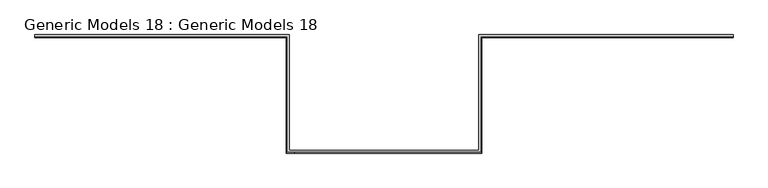
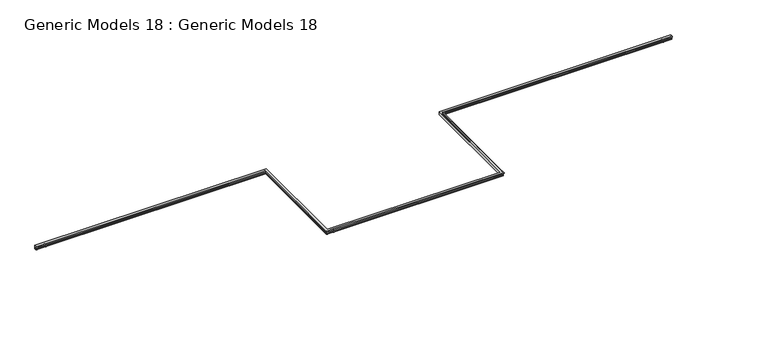
"""IFC4 building model written with IfcOpenShell, lengths in millimetres: proxy geometry, Generic Models 18 : Generic Models 18."""

from ifc_helpers import new_model, si_unit, frame, origin, place, context, project, spatial, circle_curve, ellipse_curve, source, transform, mapped, element, save
from ifc_brep_helpers import plane_surface, cylinder_surface, advanced_brep


def generic_models_18_generic_models_18_2a58dc35(model_context):
    return source(origin(), model_context, "Body", "AdvancedBrep", [
        advanced_brep(
        [(-8761.2825076, -5430.1542653, 7442.2), (-8761.2825076, -5379.3542653, 7442.2), (-8761.2825076, -5379.3542653, 7353.3), (-8761.2825076, -5417.4542653, 7353.3), (-8761.2825076, -5417.4542653, 7366.0), (-8761.2825076, -5417.4542653, 7378.7), (-8761.2825076, -5417.4542653, 7404.1), (-8761.2825076, -5417.4542653, 7416.8), (-8761.2825076, -5430.1542653, 7416.8), (-8532.6825076, -5430.1542653, 7442.2), (-3097.0825076, -5430.1542653, 7442.2), (-3097.0825076, -8034.2292912, 7442.2), (-2931.9825076, -8034.2292912, 7442.2), (1271.7174924, -8034.2292912, 7442.2), (1271.7174924, -7869.1292912, 7442.2), (1271.7174924, -5430.1542653, 7442.2), (6707.3174924, -5430.1542653, 7442.2), (6935.9174924, -5430.1542653, 7442.2), (6935.9174924, -5379.3542653, 7442.2), (1220.9174924, -5379.3542653, 7442.2), (1220.9174924, -7983.4292912, 7442.2), (-3046.2825076, -7983.4292912, 7442.2), (-3046.2825076, -5379.3542653, 7442.2), (-3046.2825076, -5379.3542653, 7353.3), (-3046.2825076, -7983.4292912, 7353.3), (1220.9174924, -7983.4292912, 7353.3), (1220.9174924, -5379.3542653, 7353.3), (6935.9174924, -5379.3542653, 7353.3), (6935.9174924, -5417.4542653, 7353.3), (6707.3174924, -5417.4542653, 7353.3), (1259.0174924, -5417.4542653, 7353.3), (1259.0174924, -7869.1292912, 7353.3), (1259.0174924, -8021.5292912, 7353.3), (-2931.9825076, -8021.5292912, 7353.3), (-3084.3825076, -8021.5292912, 7353.3), (-3084.3825076, -5417.4542653, 7353.3), (-8532.6825076, -5417.4542653, 7353.3), (-8532.6825076, -5417.4542653, 7366.0), (-3084.3825076, -5417.4542653, 7366.0), (-3084.3825076, -5417.4542653, 7378.7), (-8532.6825076, -5417.4542653, 7378.7), (-8532.6825076, -5417.4542653, 7404.1), (-3084.3825076, -5417.4542653, 7404.1), (-3084.3825076, -5417.4542653, 7416.8), (-3084.3825076, -8021.5292912, 7416.8), (1259.0174924, -8021.5292912, 7416.8), (1259.0174924, -5417.4542653, 7416.8), (6935.9174924, -5417.4542653, 7416.8), (6935.9174924, -5430.1542653, 7416.8), (6707.3174924, -5430.1542653, 7416.8), (1271.7174924, -5430.1542653, 7416.8), (1271.7174924, -7869.1292912, 7416.8), (1271.7174924, -8034.2292912, 7416.8), (-2931.9825076, -8034.2292912, 7416.8), (-3097.0825076, -8034.2292912, 7416.8), (-3097.0825076, -5430.1542653, 7416.8), (-8532.6825076, -5430.1542653, 7416.8), (-3084.3825076, -8021.5292912, 7366.0), (-3084.3825076, -8021.5292912, 7378.7), (-3084.3825076, -8021.5292912, 7404.1), (-2931.9825076, -8021.5292912, 7366.0), (1259.0174924, -8021.5292912, 7366.0), (1259.0174924, -8021.5292912, 7378.7), (-2931.9825076, -8021.5292912, 7378.7), (-2931.9825076, -8021.5292912, 7404.1), (1259.0174924, -8021.5292912, 7404.1), (1259.0174924, -7869.1292912, 7366.0), (1259.0174924, -5417.4542653, 7366.0), (1259.0174924, -5417.4542653, 7378.7), (1259.0174924, -7869.1292912, 7378.7), (1259.0174924, -7869.1292912, 7404.1), (1259.0174924, -5417.4542653, 7404.1), (6707.3174924, -5417.4542653, 7366.0), (6935.9174924, -5417.4542653, 7366.0), (6935.9174924, -5417.4542653, 7378.7), (6707.3174924, -5417.4542653, 7378.7), (6707.3174924, -5417.4542653, 7404.1), (6935.9174924, -5417.4542653, 7404.1)],
        [
            (0, 1),
            (1, 2),
            (2, 3),
            (3, 4, circle_curve(frame((-8761.2825076, -5421.1991851, 7359.65), z_axis=(-1.0, 0.0, 0.0), x_axis=(0.0, 1.0, 0.0)), 7.3720367)),
            (4, 5),
            (5, 6, circle_curve(frame((-8761.2825076, -5417.4542653, 7391.4), z_axis=(-1.0, 0.0, 0.0), x_axis=(0.0, 1.0, 0.0)), 12.7)),
            (6, 7),
            (7, 8),
            (8, 0, circle_curve(frame((-8761.2825076, -5430.1542653, 7429.5), z_axis=(-1.0, 0.0, 0.0), x_axis=(0.0, 1.0, 0.0)), 12.7)),
            (0, 9),
            (9, 10),
            (10, 11),
            (11, 12),
            (12, 13),
            (13, 14),
            (14, 15),
            (15, 16),
            (16, 17),
            (17, 18),
            (18, 19),
            (19, 20),
            (20, 21),
            (21, 22),
            (22, 1),
            (22, 23),
            (23, 2),
            (23, 24),
            (24, 25),
            (25, 26),
            (26, 27),
            (27, 28),
            (28, 29),
            (29, 30),
            (30, 31),
            (31, 32),
            (32, 33),
            (33, 34),
            (34, 35),
            (35, 36),
            (36, 3),
            (36, 37, circle_curve(frame((-8532.6825076, -5421.1991851, 7359.65), z_axis=(-1.0, 0.0, 0.0), x_axis=(0.0, 1.0, 0.0)), 7.3720367)),
            (37, 4),
            (37, 38),
            (38, 39),
            (39, 40),
            (40, 5),
            (40, 41, circle_curve(frame((-8532.6825076, -5417.4542653, 7391.4), z_axis=(-1.0, 0.0, 0.0), x_axis=(0.0, 1.0, 0.0)), 12.7)),
            (41, 6),
            (41, 42),
            (42, 43),
            (43, 7),
            (43, 44),
            (44, 45),
            (45, 46),
            (46, 47),
            (47, 48),
            (48, 49),
            (49, 50),
            (50, 51),
            (51, 52),
            (52, 53),
            (53, 54),
            (54, 55),
            (55, 56),
            (56, 8),
            (56, 9, circle_curve(frame((-8532.6825076, -5430.1542653, 7429.5), z_axis=(-1.0, 0.0, 0.0), x_axis=(0.0, 1.0, 0.0)), 12.7)),
            (35, 38, ellipse_curve(frame((-3088.1274275, -5421.1991851, 7359.65), z_axis=(-0.7071067811865458, 0.7071067811865492, 0.0), x_axis=(-0.7071067811865492, -0.7071067811865458, 0.0)), 10.4256342, 7.3720367)),
            (39, 42, ellipse_curve(frame((-3084.3825076, -5417.4542653, 7391.4), z_axis=(-0.7071067811865458, 0.7071067811865492, 0.0), x_axis=(-0.7071067811865492, -0.7071067811865458, 0.0)), 17.9605122, 12.7)),
            (55, 10, ellipse_curve(frame((-3097.0825076, -5430.1542653, 7429.5), z_axis=(-0.7071067811865458, 0.7071067811865492, 0.0), x_axis=(-0.7071067811865492, -0.7071067811865458, 0.0)), 17.9605122, 12.7)),
            (21, 24),
            (34, 57, ellipse_curve(frame((-3088.1274275, -8025.274211, 7359.65), z_axis=(-0.7071067811865468, 0.7071067811865481, 0.0), x_axis=(0.7071067811865481, 0.7071067811865469, 0.0)), 10.4256342, 7.3720367)),
            (57, 38),
            (57, 58),
            (58, 39),
            (58, 59, ellipse_curve(frame((-3084.3825076, -8021.5292912, 7391.4), z_axis=(-0.7071067811865468, 0.7071067811865481, 0.0), x_axis=(0.7071067811865481, 0.7071067811865469, 0.0)), 17.9605122, 12.7)),
            (59, 42),
            (59, 44),
            (54, 11, ellipse_curve(frame((-3097.0825076, -8034.2292912, 7429.5), z_axis=(-0.7071067811865468, 0.7071067811865481, 0.0), x_axis=(0.7071067811865481, 0.7071067811865469, 0.0)), 17.9605122, 12.7)),
            (20, 25),
            (33, 60, circle_curve(frame((-2931.9825076, -8025.274211, 7359.65), z_axis=(-1.0, 0.0, 0.0), x_axis=(0.0, 1.0, 0.0)), 7.3720367)),
            (60, 57),
            (60, 61),
            (61, 62),
            (62, 63),
            (63, 58),
            (63, 64, circle_curve(frame((-2931.9825076, -8021.5292912, 7391.4), z_axis=(-1.0, 0.0, 0.0), x_axis=(0.0, 1.0, 0.0)), 12.7)),
            (64, 59),
            (64, 65),
            (65, 45),
            (53, 12, circle_curve(frame((-2931.9825076, -8034.2292912, 7429.5), z_axis=(-1.0, 0.0, 0.0), x_axis=(0.0, 1.0, 0.0)), 12.7)),
            (32, 61, ellipse_curve(frame((1262.7624122, -8025.274211, 7359.65), z_axis=(-0.7071067811865488, -0.7071067811865461, 0.0), x_axis=(-0.7071067811865464, 0.7071067811865488, 0.0)), 10.4256342, 7.3720367)),
            (62, 65, ellipse_curve(frame((1259.0174924, -8021.5292912, 7391.4), z_axis=(-0.7071067811865488, -0.7071067811865461, 0.0), x_axis=(-0.7071067811865464, 0.7071067811865488, 0.0)), 17.9605122, 12.7)),
            (52, 13, ellipse_curve(frame((1271.7174924, -8034.2292912, 7429.5), z_axis=(-0.7071067811865488, -0.7071067811865461, 0.0), x_axis=(-0.7071067811865464, 0.7071067811865488, 0.0)), 17.9605122, 12.7)),
            (19, 26),
            (31, 66, circle_curve(frame((1262.7624122, -7869.1292912, 7359.65), z_axis=(0.0, -1.0, 0.0), x_axis=(-1.0, 0.0, 0.0)), 7.3720367)),
            (66, 61),
            (66, 67),
            (67, 68),
            (68, 69),
            (69, 62),
            (69, 70, circle_curve(frame((1259.0174924, -7869.1292912, 7391.4), z_axis=(0.0, -1.0, 0.0), x_axis=(-1.0, 0.0, 0.0)), 12.7)),
            (70, 65),
            (70, 71),
            (71, 46),
            (51, 14, circle_curve(frame((1271.7174924, -7869.1292912, 7429.5), z_axis=(0.0, -1.0, 0.0), x_axis=(-1.0, 0.0, 0.0)), 12.7)),
            (30, 67, ellipse_curve(frame((1262.7624122, -5421.1991851, 7359.65), z_axis=(-0.7071067811865492, -0.7071067811865457, 0.0), x_axis=(0.7071067811865457, -0.7071067811865493, 0.0)), 10.4256342, 7.3720367)),
            (68, 71, ellipse_curve(frame((1259.0174924, -5417.4542653, 7391.4), z_axis=(-0.7071067811865492, -0.7071067811865457, 0.0), x_axis=(0.7071067811865457, -0.7071067811865493, 0.0)), 17.9605122, 12.7)),
            (50, 15, ellipse_curve(frame((1271.7174924, -5430.1542653, 7429.5), z_axis=(-0.7071067811865492, -0.7071067811865457, 0.0), x_axis=(0.7071067811865457, -0.7071067811865493, 0.0)), 17.9605122, 12.7)),
            (18, 27),
            (29, 72, circle_curve(frame((6707.3174924, -5421.1991851, 7359.65), z_axis=(-1.0, 0.0, 0.0), x_axis=(0.0, 1.0, 0.0)), 7.3720367)),
            (72, 67),
            (72, 73),
            (73, 74),
            (74, 75),
            (75, 68),
            (75, 76, circle_curve(frame((6707.3174924, -5417.4542653, 7391.4), z_axis=(-1.0, 0.0, 0.0), x_axis=(0.0, 1.0, 0.0)), 12.7)),
            (76, 71),
            (76, 77),
            (77, 47),
            (49, 16, circle_curve(frame((6707.3174924, -5430.1542653, 7429.5), z_axis=(-1.0, 0.0, 0.0), x_axis=(0.0, 1.0, 0.0)), 12.7)),
            (17, 48, circle_curve(frame((6935.9174924, -5430.1542653, 7429.5), z_axis=(1.0, 0.0, 0.0), x_axis=(0.0, 1.0, 0.0)), 12.7)),
            (77, 74, circle_curve(frame((6935.9174924, -5417.4542653, 7391.4), z_axis=(1.0, 0.0, 0.0), x_axis=(0.0, 1.0, 0.0)), 12.7)),
            (73, 28, circle_curve(frame((6935.9174924, -5421.1991851, 7359.65), z_axis=(1.0, 0.0, 0.0), x_axis=(0.0, 1.0, 0.0)), 7.3720367)),
        ],
        [
            plane_surface(frame((-8761.2825076, -5379.3542653, 7442.2), z_axis=(-1.0, 0.0, 0.0), x_axis=(0.0, 0.0, 1.0))),
            plane_surface(frame((-8761.2825076, -5430.1542653, 7442.2), z_axis=(0.0, 0.0, 1.0), x_axis=(1.0, 0.0, 0.0))),
            plane_surface(frame((-8761.2825076, -5379.3542653, 7442.2), z_axis=(0.0, 1.0, 0.0), x_axis=(1.0, 0.0, 0.0))),
            plane_surface(frame((-8761.2825076, -5379.3542653, 7353.3), z_axis=(0.0, 0.0, -1.0), x_axis=(1.0, 0.0, 0.0))),
            cylinder_surface(frame((-8761.2825076, -5421.1991851, 7359.65), z_axis=(-1.0, 0.0, 0.0), x_axis=(0.0, 1.0, 0.0)), 7.3720367),
            plane_surface(frame((-8761.2825076, -5417.4542653, 7366.0), z_axis=(0.0, -1.0, 0.0), x_axis=(1.0, 0.0, 0.0))),
            cylinder_surface(frame((-8761.2825076, -5417.4542653, 7391.4), z_axis=(-1.0, 0.0, 0.0), x_axis=(0.0, 1.0, 0.0)), 12.7),
            plane_surface(frame((-8761.2825076, -5417.4542653, 7404.1), z_axis=(0.0, -1.0, 0.0), x_axis=(1.0, 0.0, 0.0))),
            plane_surface(frame((-8761.2825076, -5417.4542653, 7416.8), z_axis=(0.0, 0.0, -1.0), x_axis=(1.0, 0.0, 0.0))),
            cylinder_surface(frame((-8761.2825076, -5430.1542653, 7429.5), z_axis=(-1.0, 0.0, 0.0), x_axis=(0.0, 1.0, 0.0)), 12.7),
            cylinder_surface(frame((-8532.6825076, -5421.1991851, 7359.65), z_axis=(-1.0, 0.0, 0.0), x_axis=(0.0, 1.0, 0.0)), 7.3720367),
            cylinder_surface(frame((-8532.6825076, -5417.4542653, 7391.4), z_axis=(-1.0, 0.0, 0.0), x_axis=(0.0, 1.0, 0.0)), 12.7),
            cylinder_surface(frame((-8532.6825076, -5430.1542653, 7429.5), z_axis=(-1.0, 0.0, 0.0), x_axis=(0.0, 1.0, 0.0)), 12.7),
            plane_surface(frame((-3046.2825076, -5379.3542653, 7442.2), z_axis=(1.0, 0.0, 0.0), x_axis=(0.0, -1.0, 0.0))),
            cylinder_surface(frame((-3088.1274275, -5379.3542653, 7359.65), z_axis=(0.0, 1.0, 0.0), x_axis=(1.0, 0.0, 0.0)), 7.3720367),
            plane_surface(frame((-3084.3825076, -5417.4542653, 7366.0), z_axis=(-1.0, 0.0, 0.0), x_axis=(0.0, -1.0, 0.0))),
            cylinder_surface(frame((-3084.3825076, -5379.3542653, 7391.4), z_axis=(0.0, 1.0, 0.0), x_axis=(1.0, 0.0, 0.0)), 12.7),
            plane_surface(frame((-3084.3825076, -5417.4542653, 7404.1), z_axis=(-1.0, 0.0, 0.0), x_axis=(0.0, -1.0, 0.0))),
            cylinder_surface(frame((-3097.0825076, -5379.3542653, 7429.5), z_axis=(0.0, 1.0, 0.0), x_axis=(1.0, 0.0, 0.0)), 12.7),
            plane_surface(frame((-3046.2825076, -7983.4292912, 7442.2), z_axis=(0.0, 1.0, 0.0), x_axis=(1.0, 0.0, 0.0))),
            cylinder_surface(frame((-3046.2825076, -8025.274211, 7359.65), z_axis=(-1.0, 0.0, 0.0), x_axis=(0.0, 1.0, 0.0)), 7.3720367),
            plane_surface(frame((-3084.3825076, -8021.5292912, 7366.0), z_axis=(0.0, -1.0, 0.0), x_axis=(1.0, 0.0, 0.0))),
            cylinder_surface(frame((-3046.2825076, -8021.5292912, 7391.4), z_axis=(-1.0, 0.0, 0.0), x_axis=(0.0, 1.0, 0.0)), 12.7),
            plane_surface(frame((-3084.3825076, -8021.5292912, 7404.1), z_axis=(0.0, -1.0, 0.0), x_axis=(1.0, 0.0, 0.0))),
            cylinder_surface(frame((-3046.2825076, -8034.2292912, 7429.5), z_axis=(-1.0, 0.0, 0.0), x_axis=(0.0, 1.0, 0.0)), 12.7),
            cylinder_surface(frame((-2931.9825076, -8025.274211, 7359.65), z_axis=(-1.0, 0.0, 0.0), x_axis=(0.0, 1.0, 0.0)), 7.3720367),
            cylinder_surface(frame((-2931.9825076, -8021.5292912, 7391.4), z_axis=(-1.0, 0.0, 0.0), x_axis=(0.0, 1.0, 0.0)), 12.7),
            cylinder_surface(frame((-2931.9825076, -8034.2292912, 7429.5), z_axis=(-1.0, 0.0, 0.0), x_axis=(0.0, 1.0, 0.0)), 12.7),
            plane_surface(frame((1220.9174924, -7983.4292912, 7442.2), z_axis=(-1.0, 0.0, 0.0), x_axis=(0.0, 1.0, 0.0))),
            cylinder_surface(frame((1262.7624122, -7983.4292912, 7359.65), z_axis=(0.0, -1.0, 0.0), x_axis=(-1.0, 0.0, 0.0)), 7.3720367),
            plane_surface(frame((1259.0174924, -8021.5292912, 7366.0), z_axis=(1.0, 0.0, 0.0), x_axis=(0.0, 1.0, 0.0))),
            cylinder_surface(frame((1259.0174924, -7983.4292912, 7391.4), z_axis=(0.0, -1.0, 0.0), x_axis=(-1.0, 0.0, 0.0)), 12.7),
            plane_surface(frame((1259.0174924, -8021.5292912, 7404.1), z_axis=(1.0, 0.0, 0.0), x_axis=(0.0, 1.0, 0.0))),
            cylinder_surface(frame((1271.7174924, -7983.4292912, 7429.5), z_axis=(0.0, -1.0, 0.0), x_axis=(-1.0, 0.0, 0.0)), 12.7),
            cylinder_surface(frame((1262.7624122, -7869.1292912, 7359.65), z_axis=(0.0, -1.0, 0.0), x_axis=(-1.0, 0.0, 0.0)), 7.3720367),
            cylinder_surface(frame((1259.0174924, -7869.1292912, 7391.4), z_axis=(0.0, -1.0, 0.0), x_axis=(-1.0, 0.0, 0.0)), 12.7),
            cylinder_surface(frame((1271.7174924, -7869.1292912, 7429.5), z_axis=(0.0, -1.0, 0.0), x_axis=(-1.0, 0.0, 0.0)), 12.7),
            plane_surface(frame((1220.9174924, -5379.3542653, 7442.2), z_axis=(0.0, 1.0, 0.0), x_axis=(1.0, 0.0, 0.0))),
            cylinder_surface(frame((1220.9174924, -5421.1991851, 7359.65), z_axis=(-1.0, 0.0, 0.0), x_axis=(0.0, 1.0, 0.0)), 7.3720367),
            plane_surface(frame((1259.0174924, -5417.4542653, 7366.0), z_axis=(0.0, -1.0, 0.0), x_axis=(1.0, 0.0, 0.0))),
            cylinder_surface(frame((1220.9174924, -5417.4542653, 7391.4), z_axis=(-1.0, 0.0, 0.0), x_axis=(0.0, 1.0, 0.0)), 12.7),
            plane_surface(frame((1259.0174924, -5417.4542653, 7404.1), z_axis=(0.0, -1.0, 0.0), x_axis=(1.0, 0.0, 0.0))),
            cylinder_surface(frame((1220.9174924, -5430.1542653, 7429.5), z_axis=(-1.0, 0.0, 0.0), x_axis=(0.0, 1.0, 0.0)), 12.7),
            plane_surface(frame((6935.9174924, -5379.3542653, 7442.2), z_axis=(1.0, 0.0, 0.0), x_axis=(0.0, 0.0, 1.0))),
            cylinder_surface(frame((6707.3174924, -5421.1991851, 7359.65), z_axis=(-1.0, 0.0, 0.0), x_axis=(0.0, 1.0, 0.0)), 7.3720367),
            cylinder_surface(frame((6707.3174924, -5417.4542653, 7391.4), z_axis=(-1.0, 0.0, 0.0), x_axis=(0.0, 1.0, 0.0)), 12.7),
            cylinder_surface(frame((6707.3174924, -5430.1542653, 7429.5), z_axis=(-1.0, 0.0, 0.0), x_axis=(0.0, 1.0, 0.0)), 12.7),
        ],
        [
            (0, [[1, 2, 3, 4, 5, 6, 7, 8, 9]]),
            (1, [[-1, 10, 11, 12, 13, 14, 15, 16, 17, 18, 19, 20, 21, 22, 23, 24]]),
            (2, [[-2, -24, 25, 26]]),
            (3, [[-3, -26, 27, 28, 29, 30, 31, 32, 33, 34, 35, 36, 37, 38, 39, 40]]),
            (4, [[-4, -40, 41, 42]]),
            (5, [[-5, -42, 43, 44, 45, 46]]),
            (6, [[-6, -46, 47, 48]]),
            (7, [[-7, -48, 49, 50, 51]]),
            (8, [[-8, -51, 52, 53, 54, 55, 56, 57, 58, 59, 60, 61, 62, 63, 64, 65]]),
            (9, [[-9, -65, 66, -10]]),
            (10, [[-41, -39, 67, -43]]),
            (11, [[-47, -45, 68, -49]]),
            (12, [[-66, -64, 69, -11]]),
            (13, [[-25, -23, 70, -27]]),
            (14, [[-67, -38, 71, 72]]),
            (15, [[-44, -72, 73, 74]]),
            (16, [[-68, -74, 75, 76]]),
            (17, [[-50, -76, 77, -52]]),
            (18, [[-69, -63, 78, -12]]),
            (19, [[-28, -70, -22, 79]]),
            (20, [[-71, -37, 80, 81]]),
            (21, [[-73, -81, 82, 83, 84, 85]]),
            (22, [[-75, -85, 86, 87]]),
            (23, [[-53, -77, -87, 88, 89]]),
            (24, [[-78, -62, 90, -13]]),
            (25, [[-80, -36, 91, -82]]),
            (26, [[-86, -84, 92, -88]]),
            (27, [[-90, -61, 93, -14]]),
            (28, [[-29, -79, -21, 94]]),
            (29, [[-91, -35, 95, 96]]),
            (30, [[-83, -96, 97, 98, 99, 100]]),
            (31, [[-92, -100, 101, 102]]),
            (32, [[-54, -89, -102, 103, 104]]),
            (33, [[-93, -60, 105, -15]]),
            (34, [[-95, -34, 106, -97]]),
            (35, [[-101, -99, 107, -103]]),
            (36, [[-105, -59, 108, -16]]),
            (37, [[-30, -94, -20, 109]]),
            (38, [[-106, -33, 110, 111]]),
            (39, [[-98, -111, 112, 113, 114, 115]]),
            (40, [[-107, -115, 116, 117]]),
            (41, [[-55, -104, -117, 118, 119]]),
            (42, [[-108, -58, 120, -17]]),
            (43, [[121, -56, -119, 122, -113, 123, -31, -109, -19]]),
            (44, [[-110, -32, -123, -112]]),
            (45, [[-116, -114, -122, -118]]),
            (46, [[-120, -57, -121, -18]]),
        ],
    ),
    ])


if __name__ == "__main__":
    model = new_model("IFC4")
    model_context = context("Model", 3, world=origin())
    ifc_project = project(units=[si_unit("LENGTHUNIT", "METRE", prefix="MILLI")], contexts=[model_context])
    site = spatial("IfcSite", under=ifc_project)
    building = spatial("IfcBuilding", under=site)
    placement = place(None, origin())
    generic_models_18_generic_models_18_shape = generic_models_18_generic_models_18_2a58dc35(model_context)
    element("IfcBuildingElementProxy", 1, Name="Generic Models 18 : Generic Models 18", ObjectType="Generic Models 18 : Generic Models 18", at=placement, inside=building, context=model_context, shape_type="MappedRepresentation", body=[
        mapped(generic_models_18_generic_models_18_shape, transform((0.0, 0.0, 0.0), x_axis=(1.0, 0.0, 0.0), y_axis=(0.0, 1.0, 0.0), z_axis=(0.0, 0.0, 1.0))),
    ])
    save(model, "model.ifc")
